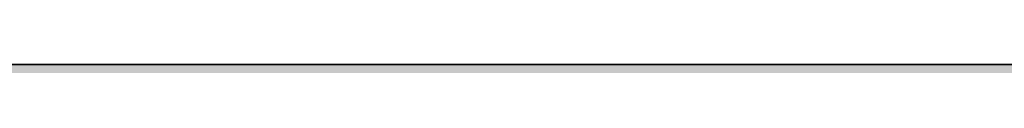
# Model space of a CAD drawing. Units: inches. Extents: x 2091 to 2899, y 967 to 2217.
# Tile 84 of 256: x 2251.24312 to 2251.2787, y 1099.91903 to 1099.91912. Entities that reach past the tile are written whole.
import ezdxf

# ---------------------------------------------------------------- set-up
doc = ezdxf.new("R2010")
doc.units = ezdxf.units.IN
doc.layers.add('A-WALL-PATT', color=141, linetype='Continuous', lineweight=13, true_color=0xadddf7)
doc.layers.add('L-SITE-WALL', color=7, linetype='Continuous', lineweight=35)

msp = doc.modelspace()

# ---------------------------------------------------------------- hatches: boundary and pattern name
at = {"layer": 'A-WALL-PATT'}
h = msp.add_hatch(color=256, dxfattribs=at)
h.dxf.hatch_style = 1
h.paths.add_polyline_path([(2212.143603, 1941.419059), (2387.643603, 1941.419059), (2387.643603, 1824.419059), (2392.143603, 1824.419059), (2392.143603, 1941.419059), (2609.643603, 1941.419059), (2609.643603, 1825.919059), (2614.143603, 1825.919059), (2614.143603, 1941.419059), (2794.143603, 1941.419059), (2794.143603, 1928.762166), (2803.143603, 1928.762166), (2803.143603, 2050.919059), (2203.143603, 2050.919059), (2203.143603, 1900.757859), (2212.143603, 1900.757859)])
h.paths.add_polyline_path([(2212.143603, 1945.919059), (2212.143603, 2041.919059), (2794.143603, 2041.919059), (2794.143603, 1945.919059), (2402.248245, 1945.919059), (2401.102434, 1945.775832), (2398.702434, 1945.775832)], flags=16)
h.paths.add_polyline_path([(2230.229861, 1948.062793), (2227.349861, 1949.502793), (2225.909861, 1951.902793), (2223.989861, 1952.862793), (2223.029861, 1955.262793), (2222.069861, 1959.582793), (2222.069861, 1963.422793), (2223.029861, 1965.662793), (2223.989861, 1965.342793), (2225.58591, 1963.860747), (2226.911533, 1964.957259), (2226.948861, 1965.938793), (2227.778319, 1966.952143), (2228.199916, 1968.878704), (2230.709861, 1964.862793), (2233.589861, 1966.302793), (2233.607309, 1966.331873), (2233.772659, 1964.938205), (2234.633802, 1963.676473), (2235.029861, 1963.902793), (2236.282035, 1965.572358), (2235.989861, 1962.942793), (2237.954512, 1957.540002), (2238.389861, 1957.902793), (2239.215861, 1960.305793), (2238.654565, 1966.38496), (2238.692792, 1966.438069), (2238.840578, 1967.499707), (2238.780291, 1967.687486), (2238.880538, 1967.786763), (2238.666861, 1966.251793), (2239.215861, 1960.305793), (2238.389861, 1957.902793), (2236.949861, 1956.702793), (2234.549861, 1949.982793)], flags=0)
h.paths.add_polyline_path([(2278.011974, 1948.062793), (2276.496427, 1947.873349), (2275.849833, 1947.688608), (2274.651974, 1947.102793)], flags=0)
h.paths.add_polyline_path([(2269.851974, 1955.742793), (2268.276176, 1956.629329), (2270.867302, 1956.348398), (2269.371974, 1958.142793), (2268.714964, 1959.192325), (2270.569833, 1958.728608), (2268.580725, 1961.906087), (2270.811974, 1960.891883), (2270.811974, 1963.422793), (2271.393315, 1964.779256), (2270.291762, 1966.156196), (2271.771974, 1965.662793), (2272.141387, 1966.524757), (2273.929833, 1965.928608), (2275.630385, 1968.054299), (2276.331938, 1966.72186), (2276.520431, 1966.952143), (2276.942029, 1968.878704), (2277.734293, 1967.611082), (2278.139888, 1969.46452), (2279.659124, 1967.033742), (2280.411974, 1966.782793), (2280.949302, 1967.588785), (2281.609833, 1967.368608), (2282.133266, 1968.153758), (2282.349235, 1966.333445), (2282.349849, 1966.332585), (2283.40755, 1968.09542), (2283.712631, 1965.52402), (2284.320221, 1964.633789), (2284.511809, 1964.889239), (2284.234974, 1965.704793), (2284.500472, 1967.318958), (2284.907944, 1965.41742), (2285.396313, 1966.068579), (2285.432833, 1966.290608), (2285.473338, 1966.171279), (2286.353919, 1967.345387), (2286.222007, 1966.158173), (2287.663492, 1968.080154), (2287.713974, 1968.442793), (2288.481599, 1969.016679), (2288.573993, 1968.728897), (2288.917461, 1969.06904), (2288.606833, 1966.837608), (2288.928726, 1963.35131), (2288.934974, 1963.356793), (2288.929731, 1963.340422), (2289.015281, 1962.413869), (2290.111223, 1963.875126), (2290.132833, 1963.942608), (2290.217672, 1964.017058), (2290.111223, 1963.875126), (2289.155833, 1960.891608), (2288.594036, 1959.257227), (2288.571974, 1959.102793), (2289.531974, 1960.542793), (2290.011974, 1962.462793), (2290.19184, 1962.642659), (2289.769833, 1959.688608), (2286.889833, 1957.288608), (2284.489833, 1950.568608), (2283.314658, 1950.046308), (2283.291974, 1949.982793), (2280.290059, 1948.648608), (2281.129833, 1948.648608), (2282.569833, 1948.168608), (2283.204726, 1948.062793), (2278.971974, 1948.062793), (2276.091974, 1949.502793), (2274.651974, 1951.902793), (2272.731974, 1952.862793)], flags=0)
h.paths.add_polyline_path([(2271.158868, 1958.021765), (2272.969833, 1955.848608), (2272.009833, 1960.168608), (2272.009833, 1964.008608), (2272.624426, 1965.442658), (2274.328023, 1963.860747), (2275.653646, 1964.957259), (2275.637743, 1964.53909), (2277.412231, 1966.006888), (2277.032974, 1965.156793), (2276.829924, 1964.975597), (2276.766012, 1963.295014), (2277.449635, 1962.66022), (2279.451974, 1964.862793), (2282.331974, 1966.302793), (2283.529833, 1966.888608), (2283.294512, 1966.770948), (2283.912993, 1963.8847), (2284.899249, 1964.448275), (2284.731974, 1962.942793), (2286.696625, 1957.540002), (2287.131974, 1957.902793), (2287.541913, 1959.095388), (2287.779395, 1958.442311), (2285.682738, 1956.695097), (2285.876503, 1959.795336), (2284.731974, 1962.942793), (2284.899249, 1964.448275), (2283.912993, 1963.8847), (2284.223833, 1962.434116), (2283.424365, 1963.605484), (2281.609833, 1962.568608), (2281.129833, 1960.168608), (2282.089833, 1956.328608), (2283.049833, 1952.968608), (2282.569833, 1950.568608), (2280.169833, 1948.648608), (2279.883316, 1948.791867), (2278.971974, 1948.062793), (2278.971974, 1949.022793), (2278.672313, 1949.397368), (2277.289833, 1950.088608), (2275.849833, 1952.488608), (2273.929833, 1953.448608), (2272.489833, 1954.888608), (2271.921647, 1954.888608), (2271.771974, 1955.262793)], flags=0)
h.paths.add_polyline_path([(2311.994146, 1955.742793), (2312.062717, 1955.674221), (2312.0551, 1955.7085)], flags=0)
h.paths.add_polyline_path([(2331.956146, 1963.951793), (2333.396146, 1965.391793), (2331.077146, 1963.356793), (2330.998603, 1963.111517)], flags=0)
h.paths.add_polyline_path([(2310.554146, 1954.302793), (2307.039807, 1956.279943), (2310.762903, 1955.876284), (2312.474146, 1953.822793), (2313.434146, 1951.422793), (2315.354146, 1950.462793), (2316.794146, 1948.062793), (2317.466146, 1947.726793), (2319.368691, 1947.964611), (2317.754146, 1949.982793), (2317.569531, 1950.610485), (2316.794146, 1951.902793), (2314.874146, 1952.862793), (2313.914146, 1955.262793), (2311.514146, 1958.142793), (2309.375489, 1961.559168), (2311.514146, 1960.337078), (2311.514146, 1961.982793), (2310.604672, 1963.119635), (2311.726605, 1962.47853), (2312.418332, 1964.09256), (2312.255964, 1964.29552), (2313.194146, 1963.982793), (2313.914146, 1965.662793), (2314.646778, 1965.418582), (2315.354146, 1966.302793), (2316.794146, 1967.742793), (2316.157435, 1966.946904), (2317.034111, 1965.28186), (2317.222604, 1965.512143), (2317.777048, 1968.045771), (2318.474111, 1966.72186), (2318.662604, 1966.952143), (2319.084201, 1968.878704), (2321.207049, 1965.482147), (2322.161419, 1966.913702), (2322.554146, 1966.782793), (2322.785988, 1967.130555), (2322.881646, 1966.324293), (2323.312041, 1965.72174), (2323.651289, 1965.891364), (2324.3965, 1967.133382), (2324.656945, 1964.938205), (2324.971986, 1964.476611), (2325.38728, 1967.001499), (2325.940813, 1964.418348), (2327.228929, 1966.135836), (2327.16632, 1965.572358), (2328.059139, 1966.762783), (2328.224576, 1966.247486), (2329.667971, 1967.67691), (2329.664576, 1967.687486), (2329.764823, 1967.786763), (2329.551146, 1966.251793), (2330.100146, 1960.305793), (2329.332814, 1958.07347), (2329.313065, 1957.935225), (2329.634146, 1958.202793), (2330.234146, 1959.102793), (2330.714146, 1961.022793), (2331.034146, 1961.342793), (2330.714146, 1959.102793), (2329.634146, 1958.202793), (2329.274146, 1957.662793), (2327.712112, 1956.361098), (2325.434146, 1949.982793), (2324.333769, 1949.493736), (2323.994146, 1948.542793), (2319.674146, 1946.622793), (2316.794146, 1948.062793), (2315.354146, 1950.462793), (2313.434146, 1951.422793)], flags=0)
h.paths.add_polyline_path([(2321.335684, 1947.952023), (2321.114146, 1948.062793), (2321.114146, 1949.022793), (2319.194146, 1951.422793), (2316.794146, 1959.582793), (2316.663237, 1959.582793), (2315.354146, 1958.142793), (2314.394146, 1958.142793), (2313.148303, 1958.709085), (2312.954146, 1959.582793), (2312.954146, 1960.891883), (2315.834146, 1959.582793), (2316.663237, 1959.582793), (2317.314709, 1960.299412), (2315.030195, 1962.420747), (2316.355818, 1963.517259), (2316.372337, 1963.951615), (2316.470195, 1963.860747), (2317.795818, 1964.957259), (2317.755219, 1963.889687), (2319.175146, 1965.156793), (2319.498407, 1965.881372), (2321.114146, 1965.342793), (2323.235885, 1962.372358), (2325.686349, 1963.772623), (2325.542789, 1962.480576), (2325.198783, 1963.494014), (2324.47851, 1963.082429), (2324.926005, 1960.994116), (2324.078087, 1962.236473), (2322.414791, 1961.286018), (2322.074146, 1959.582793), (2323.034146, 1955.742793), (2323.994146, 1952.382793), (2323.514146, 1949.982793), (2322.142717, 1948.88565), (2322.074146, 1948.542793)], flags=0)
h.paths.add_polyline_path([(2320.207479, 1963.337459), (2320.154146, 1963.422793), (2320.394146, 1963.542793)], flags=0)
h.paths.add_polyline_path([(2353.850527, 1965.8105), (2354.030527, 1965.7505), (2354.330527, 1966.4505), (2354.330527, 1966.9305)], flags=0)
h.paths.add_polyline_path([(2359.020582, 1969.026412), (2359.098382, 1968.901932), (2359.233527, 1969.5195), (2359.233527, 1969.9995)], flags=0)
h.paths.add_polyline_path([(2358.256694, 1966.681672), (2357.983601, 1966.348035), (2358.211267, 1966.146175), (2358.410492, 1966.389568)], flags=0)
h.paths.add_polyline_path([(2357.768473, 1966.058778), (2357.7322, 1965.104967), (2357.751047, 1965.120556), (2357.769527, 1965.6065), (2357.769527, 1966.057843)], flags=0)
h.paths.add_polyline_path([(2359.111527, 1965.3045), (2359.111527, 1964.8245), (2359.844527, 1966.4675), (2359.844527, 1966.9475)], flags=0)
h.paths.add_polyline_path([(2360.223684, 1966.621449), (2360.698527, 1969.3625), (2360.698527, 1969.8425), (2360.210527, 1967.0255), (2360.210527, 1966.6425)], flags=0)
h.paths.add_polyline_path([(2363.450527, 1967.8905), (2363.450527, 1968.3705), (2362.490527, 1966.9305), (2362.656045, 1966.698776)], flags=0)
h.paths.add_polyline_path([(2364.475523, 1966.078826), (2365.850527, 1968.3705), (2365.850527, 1968.8505), (2364.427975, 1966.479581)], flags=0)
h.paths.add_polyline_path([(2366.313527, 1965.8525), (2366.366709, 1965.695829), (2366.802527, 1968.3455), (2366.802527, 1968.8255)], flags=0)
h.paths.add_polyline_path([(2367.16531, 1965.803544), (2367.290527, 1966.9305), (2367.290527, 1967.4105), (2367.102701, 1965.720066)], flags=0)
h.paths.add_polyline_path([(2370.036527, 1959.9735), (2371.013527, 1963.0245), (2371.013527, 1963.5045), (2370.036527, 1960.4535)], flags=0)
h.paths.add_polyline_path([(2371.610527, 1960.2105), (2372.570527, 1961.6505), (2372.570527, 1962.1305), (2371.802527, 1960.9785)], flags=0)
h.paths.add_polyline_path([(2350.873666, 1956.005086), (2351.930527, 1955.8905), (2354.490527, 1953.3305), (2353.850527, 1954.9305), (2351.450527, 1957.8105), (2347.935527, 1963.4255), (2347.935527, 1963.9055), (2351.450527, 1958.2905), (2353.705073, 1955.585046), (2352.890527, 1959.2505), (2352.890527, 1959.7305), (2352.890527, 1961.924786), (2356.730527, 1959.7305), (2358.454471, 1961.626838), (2354.810527, 1965.0105), (2355.030855, 1965.28591), (2358.691091, 1961.88712), (2361.530527, 1965.0105), (2364.376495, 1966.433484), (2364.524394, 1965.186911), (2365.454468, 1963.824181), (2365.881073, 1964.067955), (2365.370527, 1966.4505), (2365.370527, 1966.9305), (2366.810527, 1960.2105), (2366.810527, 1959.7305), (2366.388709, 1952.981409), (2367.770527, 1956.8505), (2368.641225, 1957.576082), (2366.810527, 1962.6105), (2366.810527, 1963.0905), (2368.775179, 1957.68771), (2369.210527, 1958.0505), (2370.001592, 1960.351867), (2369.475232, 1966.052668), (2369.513458, 1966.105777), (2369.514173, 1966.110912), (2369.475232, 1966.532668), (2369.513458, 1966.585777), (2369.614635, 1967.312591), (2369.182527, 1968.6585), (2369.182527, 1969.1385), (2369.600957, 1967.835194), (2369.701204, 1967.934471), (2369.717947, 1968.054743), (2370.145176, 1968.374145), (2369.778707, 1968.011224), (2369.701204, 1967.454471), (2370.468161, 1968.214004), (2369.674936, 1967.265771), (2369.514173, 1966.110912), (2370.036527, 1960.4535), (2370.036527, 1959.9735), (2369.441756, 1958.243191), (2370.650527, 1959.2505), (2371.045821, 1962.017559), (2371.130527, 1962.1305), (2370.650527, 1958.7705), (2367.770527, 1956.3705), (2365.370527, 1949.6505), (2362.079099, 1948.187643), (2363.450527, 1947.7305), (2361.050527, 1947.7305), (2360.090527, 1947.7305), (2357.103861, 1947.357167), (2360.090527, 1948.2105), (2358.170527, 1949.1705), (2356.730527, 1951.5705), (2354.810527, 1952.5305), (2351.930527, 1955.4105)], flags=0)
h.paths.add_polyline_path([(2361.050527, 1948.6905), (2359.130527, 1951.0905), (2356.730527, 1959.2505), (2355.770527, 1959.2505), (2352.890527, 1960.559591), (2352.890527, 1961.444786), (2355.890527, 1959.7305), (2356.730527, 1959.7305), (2356.837194, 1959.367834), (2361.530527, 1964.5305), (2363.248422, 1965.389448), (2364.92531, 1963.041805), (2362.490527, 1961.6505), (2362.063861, 1959.517167), (2362.970527, 1955.8905), (2363.930527, 1952.5305), (2363.930527, 1952.0505), (2363.450527, 1949.6505), (2361.050527, 1947.7305)], flags=0)
h.paths.add_polyline_path([(2359.130527, 1951.5705), (2359.290527, 1951.3705), (2361.050527, 1954.4505), (2361.050527, 1954.9305)], flags=0)
h.paths.add_polyline_path([(2357.219527, 1966.5455), (2356.792527, 1968.8145), (2356.792527, 1969.2945), (2357.219527, 1967.0255)], flags=0)
h.paths.add_polyline_path([(2361.050527, 1954.4505), (2361.530527, 1958.7705), (2361.530527, 1959.2505), (2361.050527, 1954.9305)], flags=0)
h.paths.add_polyline_path([(2402.548287, 1948.486076), (2402.302434, 1948.415832), (2402.590434, 1948.415832)], flags=0)
h.paths.add_polyline_path([(2394.142434, 1956.095832), (2395.685052, 1954.553214), (2396.720495, 1953.970679), (2396.062434, 1955.615832), (2395.241381, 1956.601096), (2395.878904, 1956.441715), (2395.102434, 1959.935832), (2395.102434, 1963.775832), (2396.062434, 1966.015832), (2397.022434, 1965.695832), (2398.618483, 1964.213787), (2399.944106, 1965.310299), (2399.981434, 1966.291832), (2400.810891, 1967.305183), (2401.232489, 1969.231744), (2403.537949, 1965.543008), (2403.941984, 1967.389316), (2404.702434, 1967.135832), (2405.460328, 1966.07478), (2406.622434, 1966.655832), (2406.639882, 1966.684913), (2406.805232, 1965.291245), (2406.925694, 1965.114746), (2407.342434, 1964.975832), (2407.874326, 1965.77367), (2408.1691, 1964.398055), (2409.314608, 1965.925398), (2409.217458, 1965.051054), (2409.445232, 1963.131245), (2410.306374, 1961.869513), (2410.702434, 1962.095832), (2411.442269, 1963.082279), (2411.165434, 1963.897832), (2411.616426, 1966.639757), (2411.725365, 1966.791109), (2411.873151, 1967.852747), (2411.812864, 1968.040526), (2411.913111, 1968.139803), (2411.699434, 1966.604832), (2412.248434, 1960.658832), (2413.225434, 1963.709832), (2414.3779, 1964.72116), (2414.513151, 1965.692747), (2414.452864, 1965.880526), (2414.553111, 1965.979803), (2414.3779, 1964.72116), (2414.519817, 1964.845697), (2414.365365, 1964.631109), (2414.339434, 1964.444832), (2414.888434, 1958.498832), (2414.062434, 1956.095832), (2412.622434, 1954.895832), (2410.17137, 1948.032854), (2410.016719, 1948.084404), (2405.902434, 1946.255832), (2405.902434, 1947.215832), (2405.204252, 1948.08856), (2404.222434, 1948.415832), (2403.262434, 1948.415832), (2400.382434, 1949.855832), (2399.662434, 1951.055832), (2397.982434, 1952.735832), (2397.022434, 1953.215832), (2395.685052, 1954.553214), (2392.656776, 1956.256908)], flags=0)
h.paths.add_polyline_path([(2409.08565, 1964.407441), (2409.130363, 1964.275715), (2409.262434, 1964.495832)], flags=0)
h.paths.add_polyline_path([(2397.742434, 1961.615832), (2398.702434, 1963.855832), (2399.662434, 1963.535832), (2401.426563, 1965.740994), (2401.791415, 1966.5588), (2402.071434, 1965.070832), (2402.835507, 1964.393367), (2403.262398, 1964.9149), (2403.338119, 1964.771086), (2402.615516, 1963.976223), (2402.498612, 1960.902238), (2403.542997, 1959.932452), (2404.413203, 1960.889679), (2404.702434, 1962.335832), (2407.916347, 1964.172354), (2409.520211, 1961.926944), (2410.987085, 1957.893042), (2411.422434, 1958.255832), (2412.047964, 1960.075625), (2412.410341, 1959.079088), (2411.675621, 1958.466821), (2411.662434, 1958.255832), (2411.62607, 1958.425529), (2409.982434, 1957.055832), (2407.582434, 1950.335832), (2403.262434, 1948.415832), (2403.262434, 1949.375832), (2401.342434, 1951.775832), (2399.416508, 1958.323981), (2397.742434, 1959.084923), (2397.742434, 1959.970118), (2397.102434, 1960.335832), (2397.742434, 1960.044923)], flags=0)
h.paths.add_polyline_path([(2405.902434, 1952.975832), (2405.950434, 1953.407832), (2406.016719, 1953.175832)], flags=0)
h.paths.add_polyline_path([(2449.817778, 1967.114014), (2449.752323, 1967.135832), (2449.793703, 1967.077901)], flags=0)
h.paths.add_polyline_path([(2451.697696, 1966.61812), (2451.740895, 1966.690118), (2451.692051, 1966.665696)], flags=0)
h.paths.add_polyline_path([(2454.343628, 1965.737572), (2455.752323, 1967.615832), (2455.992323, 1968.095832), (2454.364497, 1965.925398)], flags=0)
h.paths.add_polyline_path([(2457.547323, 1968.863832), (2457.787323, 1969.343832), (2457.054323, 1968.795832), (2457.007622, 1968.460345)], flags=0)
h.paths.add_polyline_path([(2456.921784, 1967.856662), (2456.802238, 1968.229016), (2456.723, 1967.659803)], flags=0)
h.paths.add_polyline_path([(2457.302323, 1967.376832), (2457.542323, 1967.856832), (2456.810323, 1966.839832), (2456.740516, 1966.700218), (2456.749021, 1966.608105)], flags=0)
h.paths.add_polyline_path([(2458.275323, 1963.709832), (2458.155343, 1963.335153), (2460.354323, 1965.264832), (2460.594323, 1965.744832)], flags=0)
h.paths.add_polyline_path([(2458.392323, 1962.815832), (2458.364088, 1962.618185), (2459.592323, 1964.255832), (2459.832323, 1964.735832)], flags=0)
h.paths.add_polyline_path([(2459.352323, 1962.815832), (2459.272323, 1962.495832), (2460.072323, 1963.295832), (2460.312323, 1963.775832)], flags=0)
h.paths.add_polyline_path([(2458.680323, 1960.607832), (2458.632323, 1960.415832), (2459.592323, 1961.855832), (2459.832323, 1962.335832)], flags=0)
h.paths.add_polyline_path([(2437.83817, 1956.24265), (2439.192323, 1956.095832), (2441.352323, 1953.935832), (2440.872323, 1955.135832), (2438.472323, 1958.015832), (2438.071563, 1958.656023), (2438.712323, 1958.495832), (2440.639596, 1956.183105), (2439.912323, 1959.455832), (2439.912323, 1963.295832), (2441.352323, 1966.655832), (2441.592323, 1967.135832), (2441.112323, 1966.015832), (2442.072323, 1965.695832), (2443.988993, 1968.09167), (2444.241323, 1966.750832), (2444.916801, 1966.15192), (2445.676574, 1967.080136), (2446.255323, 1969.724832), (2446.495323, 1970.204832), (2446.282379, 1969.231744), (2447.362672, 1967.503275), (2447.720323, 1969.567832), (2447.960323, 1970.047832), (2447.48548, 1967.306781), (2448.792323, 1965.215832), (2448.472323, 1964.863832), (2448.552323, 1964.735832), (2451.452051, 1966.185696), (2451.615122, 1964.811245), (2452.307917, 1963.796172), (2453.234505, 1964.325651), (2454.072323, 1960.415832), (2453.628687, 1953.317651), (2454.792323, 1956.575832), (2455.032323, 1957.055832), (2455.718835, 1957.627926), (2453.832323, 1962.815832), (2453.940966, 1963.793615), (2453.335323, 1965.577832), (2453.824323, 1968.550832), (2454.064323, 1969.030832), (2453.575323, 1966.057832), (2454.040333, 1964.687919), (2453.832323, 1962.815832), (2455.718835, 1957.627926), (2456.367207, 1958.168235), (2457.058323, 1960.178832), (2457.298323, 1960.658832), (2456.472323, 1958.255832), (2457.717729, 1959.29367), (2457.672323, 1958.975832), (2454.889951, 1956.657188), (2453.614142, 1953.084923), (2453.592323, 1952.735832), (2453.352323, 1952.255832), (2453.359596, 1952.372196), (2452.632323, 1950.335832), (2452.392323, 1949.855832), (2449.203752, 1948.43869), (2450.712323, 1947.935832), (2448.072323, 1947.935832), (2447.112323, 1947.935832), (2444.552323, 1947.615832), (2447.199596, 1948.372196), (2445.192323, 1949.375832), (2443.752323, 1951.775832), (2441.832323, 1952.735832), (2438.952323, 1955.615832)], flags=0)
h.paths.add_polyline_path([(2443.992323, 1959.935832), (2444.040323, 1959.772632), (2444.121554, 1959.861986)], flags=0)
h.paths.add_polyline_path([(2442.912323, 1959.935832), (2443.032323, 1959.935832), (2442.445657, 1960.202499)], flags=0)
h.paths.add_polyline_path([(2444.982943, 1965.019677), (2445.279323, 1965.264832), (2445.519323, 1965.744832), (2444.993996, 1965.310299)], flags=0)
h.paths.add_polyline_path([(2446.133323, 1965.029832), (2446.330366, 1965.471499), (2444.970323, 1964.257832), (2444.730323, 1963.777832)], flags=0)
h.paths.add_polyline_path([(2442.792323, 1959.455832), (2443.752323, 1959.455832), (2446.152323, 1951.295832), (2446.412323, 1951.750832), (2446.392323, 1951.775832), (2448.080599, 1954.730315), (2448.552323, 1958.975832), (2441.832323, 1965.215832), (2442.154946, 1965.619111), (2448.792323, 1959.455832), (2448.312323, 1955.135832), (2448.072323, 1954.655832), (2446.412323, 1951.750832), (2448.312323, 1949.375832), (2448.312323, 1948.415832), (2450.540895, 1950.19869), (2450.952323, 1952.255832), (2449.992323, 1955.615832), (2449.032323, 1959.455832), (2449.512323, 1961.855832), (2449.752323, 1962.335832), (2449.674904, 1961.948736), (2452.994505, 1963.845651), (2453.064414, 1963.519409), (2452.884611, 1963.782854), (2449.674904, 1961.948736), (2449.272323, 1959.935832), (2450.232323, 1956.095832), (2451.192323, 1952.735832), (2450.712323, 1950.335832), (2450.472323, 1949.855832), (2448.072323, 1947.935832), (2448.072323, 1948.535832), (2445.432323, 1949.855832), (2443.992323, 1952.255832), (2442.072323, 1953.215832), (2441.112323, 1955.615832), (2440.152323, 1959.935832), (2440.152323, 1960.655832)], flags=0)
h.paths.add_polyline_path([(2456.692323, 1966.985832), (2457.608323, 1968.080832), (2457.848323, 1968.560832), (2456.932323, 1967.465832)], flags=0)
h.paths.add_polyline_path([(2489.89657, 1966.580241), (2489.942948, 1966.189347), (2490.747488, 1967.530248), (2491.319122, 1968.951161)], flags=0)
h.paths.add_polyline_path([(2473.562471, 1956.407131), (2477.139981, 1956.019257), (2476.955333, 1956.240834), (2475.108049, 1957.280108), (2476.347488, 1956.970248), (2475.186901, 1958.824216), (2476.919122, 1958.391161), (2475.411642, 1960.799269), (2477.787488, 1959.719339), (2477.787488, 1962.250248), (2477.637399, 1962.43786), (2477.82255, 1962.332059), (2478.359122, 1963.58406), (2478.359122, 1963.671161), (2477.324348, 1964.964628), (2478.714826, 1964.501135), (2479.319122, 1965.911161), (2480.279122, 1965.591161), (2481.783965, 1967.472214), (2482.116488, 1965.705248), (2482.880562, 1965.027782), (2483.209305, 1965.429408), (2483.220169, 1965.71509), (2483.07594, 1965.989022), (2483.711762, 1966.765808), (2484.130488, 1968.679248), (2484.702122, 1970.100161), (2484.489177, 1969.127072), (2486.502904, 1965.905109), (2487.387488, 1965.610248), (2488.153419, 1966.759144), (2488.717017, 1965.970108), (2489.200086, 1966.211642), (2489.330671, 1965.110992), (2490.393905, 1963.622465), (2490.660765, 1963.774956), (2490.493905, 1964.553636), (2490.923063, 1963.924841), (2491.319122, 1964.151161), (2491.333389, 1964.170183), (2491.210488, 1964.532248), (2491.281756, 1964.965537), (2491.425789, 1964.293383), (2494.076476, 1967.827632), (2494.497918, 1966.514942), (2494.598165, 1966.614218), (2494.689488, 1967.270248), (2495.106748, 1967.582196), (2495.129839, 1967.748075), (2495.069552, 1967.935854), (2495.169799, 1968.035131), (2495.031777, 1967.043632), (2495.753818, 1967.758684), (2494.982053, 1966.686437), (2494.956122, 1966.500161), (2495.479021, 1960.836851), (2495.910488, 1962.184248), (2496.482122, 1963.605161), (2496.072694, 1962.326589), (2496.768904, 1962.937536), (2496.599122, 1962.711161), (2496.119122, 1959.351161), (2496.732873, 1960.271787), (2496.987488, 1961.290248), (2497.559122, 1962.711161), (2497.079122, 1960.791161), (2496.507488, 1959.370248), (2495.547488, 1957.930248), (2492.758842, 1955.606376), (2490.839122, 1950.231161), (2490.267488, 1948.810248), (2485.947488, 1946.890248), (2483.067488, 1948.330248), (2481.627488, 1950.730248), (2479.707488, 1951.690248), (2476.827488, 1954.570248)], flags=0)
h.paths.add_polyline_path([(2485.576973, 1948.313392), (2485.559122, 1948.311161), (2485.578758, 1948.311161)], flags=0)
h.paths.add_polyline_path([(2478.645063, 1954.551161), (2478.109042, 1956.963257), (2479.319122, 1955.511161), (2480.279122, 1953.111161), (2482.199122, 1952.151161), (2483.639122, 1949.751161), (2486.519122, 1948.311161), (2486.519122, 1949.271161), (2484.739307, 1951.49593), (2484.027488, 1950.250248), (2481.627488, 1958.410248), (2482.375148, 1959.232673), (2482.199122, 1959.831161), (2483.197572, 1960.929456), (2479.707488, 1964.170248), (2480.603358, 1965.290085), (2481.875171, 1964.109115), (2482.666387, 1964.763582), (2482.615359, 1963.421798), (2482.989199, 1963.074661), (2484.008488, 1963.984248), (2484.683606, 1965.497507), (2484.580122, 1965.405161), (2485.357268, 1967.147113), (2485.120645, 1965.781197), (2486.427488, 1963.690248), (2488.145383, 1964.549195), (2489.822271, 1962.201552), (2490.747488, 1962.730248), (2491.999662, 1964.399813), (2492.076046, 1965.087265), (2492.212892, 1964.684119), (2492.485374, 1965.047429), (2492.279122, 1963.191161), (2494.243773, 1957.78837), (2494.562503, 1958.053978), (2494.933488, 1959.133248), (2495.505122, 1960.554161), (2494.679122, 1958.151161), (2494.107488, 1956.730248), (2494.562503, 1958.053978), (2493.408544, 1957.092345), (2491.707488, 1961.770248), (2491.999662, 1964.399813), (2490.747488, 1962.730248), (2487.71203, 1960.9957), (2487.479122, 1959.831161), (2488.439122, 1955.991161), (2489.399122, 1952.631161), (2488.919122, 1950.231161), (2488.576918, 1949.957397), (2488.347488, 1948.810248), (2487.651715, 1948.253629), (2487.479122, 1948.311161), (2486.519122, 1948.311161), (2483.639122, 1949.751161), (2482.199122, 1952.151161), (2480.279122, 1953.111161), (2478.839122, 1954.551161)], flags=0)
h.paths.add_polyline_path([(2526.648252, 1966.987524), (2526.517343, 1967.031161), (2526.600102, 1966.915298)], flags=0)
h.paths.add_polyline_path([(2528.47064, 1966.446656), (2528.574486, 1966.619732), (2528.457071, 1966.561025)], flags=0)
h.paths.add_polyline_path([(2534.133343, 1967.496161), (2534.156685, 1967.542845), (2534.059841, 1967.408296)], flags=0)
h.paths.add_polyline_path([(2536.161923, 1964.0506), (2535.157343, 1962.711161), (2535.100872, 1962.315866), (2536.117343, 1963.671161), (2536.420532, 1964.277539)], flags=0)
h.paths.add_polyline_path([(2535.157343, 1959.831161), (2536.117343, 1961.271161), (2536.597343, 1962.231161), (2535.253343, 1960.215161)], flags=0)
h.paths.add_polyline_path([(2513.249035, 1956.284796), (2516.221181, 1955.962555), (2514.997343, 1957.431161), (2514.195823, 1958.711541), (2515.477343, 1958.391161), (2516.931888, 1956.645706), (2516.437343, 1958.871161), (2516.437343, 1962.711161), (2516.872692, 1963.726974), (2515.346434, 1965.634797), (2517.397343, 1964.951161), (2517.877343, 1966.071161), (2518.357343, 1967.031161), (2517.877343, 1965.911161), (2518.837343, 1965.591161), (2520.48659, 1967.652719), (2520.766343, 1966.166161), (2521.530417, 1965.488695), (2521.781443, 1965.795375), (2521.800911, 1966.307268), (2521.477804, 1966.920936), (2521.246343, 1967.126161), (2521.177701, 1967.490913), (2521.477804, 1966.920936), (2522.010417, 1966.448695), (2522.257386, 1966.750417), (2522.780343, 1969.140161), (2523.260343, 1970.100161), (2523.047398, 1969.127072), (2524.673132, 1966.525897), (2526.037343, 1966.071161), (2526.795238, 1965.010108), (2527.977071, 1965.601025), (2528.140141, 1964.226573), (2528.66459, 1963.458159), (2529.388616, 1963.871888), (2529.329665, 1964.14699), (2529.481284, 1963.924841), (2529.877343, 1964.151161), (2529.98401, 1964.293383), (2529.789053, 1965.20318), (2530.0624, 1964.397903), (2532.802483, 1968.051347), (2533.147773, 1966.975854), (2533.24802, 1967.075131), (2533.339343, 1967.731161), (2533.672848, 1967.980493), (2533.72802, 1968.035131), (2533.514343, 1966.500161), (2534.024718, 1960.972496), (2534.560343, 1962.645161), (2535.040343, 1963.605161), (2534.063343, 1960.554161), (2533.237343, 1958.151161), (2534.288154, 1959.026836), (2534.197343, 1958.391161), (2531.512597, 1956.153872), (2529.397343, 1950.231161), (2528.917343, 1949.271161), (2526.448772, 1948.174018), (2527.477343, 1947.831161), (2530.357343, 1947.351161), (2524.597343, 1947.351161), (2521.717343, 1948.791161), (2520.277343, 1951.191161), (2518.357343, 1952.151161), (2515.477343, 1955.031161)], flags=0)
h.paths.add_polyline_path([(2523.93476, 1967.190308), (2523.619512, 1966.483689), (2523.7705, 1966.242109)], flags=0)
h.paths.add_polyline_path([(2518.837343, 1953.111161), (2517.877343, 1955.511161), (2516.884983, 1959.976779), (2516.917343, 1959.96207), (2516.917343, 1962.025446), (2520.757343, 1959.831161), (2522.024949, 1961.225527), (2518.357343, 1964.631161), (2519.002589, 1965.437718), (2520.433392, 1964.109115), (2521.30112, 1964.826871), (2521.245157, 1963.355333), (2525.638307, 1959.27598), (2526.037343, 1961.271161), (2529.397343, 1963.191161), (2530.649517, 1964.860726), (2530.66472, 1964.99755), (2530.691956, 1964.917311), (2531.087778, 1965.445074), (2530.945985, 1964.168944), (2530.691956, 1964.917311), (2529.397343, 1963.191161), (2526.362504, 1961.456967), (2526.037343, 1959.831161), (2526.997343, 1955.991161), (2527.957343, 1952.631161), (2527.477343, 1950.231161), (2527.134486, 1949.956875), (2526.973928, 1949.154087), (2526.697343, 1949.031161), (2524.597343, 1947.351161), (2524.597343, 1948.311161), (2524.277343, 1948.711161), (2522.197343, 1949.751161), (2520.757343, 1952.151161)], flags=0)
h.paths.add_polyline_path([(2520.277343, 1958.871161), (2520.853343, 1959.504761), (2523.157343, 1951.671161), (2524.613895, 1954.220126), (2524.597343, 1954.071161), (2522.677343, 1950.711161)], flags=0)
h.paths.add_polyline_path([(2559.37091, 1966.311161), (2559.398411, 1966.324911), (2559.401943, 1966.345296)], flags=0)
h.paths.add_polyline_path([(2549.77091, 1957.191161), (2552.65091, 1954.311161), (2552.133987, 1955.603468), (2550.61091, 1957.431161), (2547.09591, 1963.046161), (2545.77591, 1965.206161), (2549.29091, 1959.591161), (2551.69091, 1956.711161), (2550.792933, 1960.752059), (2550.73091, 1960.780251), (2550.73091, 1964.871161), (2551.69091, 1967.111161), (2552.65091, 1966.791161), (2554.246959, 1965.309115), (2555.034252, 1965.960337), (2555.581671, 1966.644612), (2555.60991, 1967.387161), (2556.439368, 1968.400511), (2556.860966, 1970.327072), (2559.37091, 1966.311161), (2560.69091, 1964.151161), (2562.408805, 1965.010108), (2561.65091, 1966.071161), (2560.33091, 1968.231161), (2561.758497, 1966.23254), (2562.347213, 1967.115614), (2562.433709, 1966.386573), (2563.127798, 1965.369604), (2563.57091, 1965.591161), (2563.588359, 1965.620241), (2563.362543, 1967.52354), (2563.722489, 1965.843792), (2565.060001, 1968.072979), (2564.732862, 1965.128722), (2565.117577, 1963.333383), (2567.444622, 1966.436109), (2567.315615, 1967.833328), (2567.353841, 1967.886437), (2567.501627, 1968.948075), (2567.44134, 1969.135854), (2567.541587, 1969.235131), (2567.32791, 1967.700161), (2567.87691, 1961.754161), (2568.746689, 1964.470327), (2568.635615, 1965.673328), (2568.673841, 1965.726437), (2568.821627, 1966.788075), (2568.76134, 1966.975854), (2568.861587, 1967.075131), (2568.64791, 1965.540161), (2568.726127, 1964.693026), (2568.85391, 1964.805161), (2568.746689, 1964.470327), (2568.817236, 1963.706261), (2568.97091, 1963.911161), (2568.866075, 1963.17731), (2569.19691, 1959.594161), (2568.37091, 1957.191161), (2566.93091, 1955.991161), (2564.620272, 1949.521373), (2564.65091, 1949.511161), (2564.616625, 1949.511161), (2564.53091, 1949.271161), (2560.21091, 1947.351161), (2557.33091, 1948.791161), (2556.045196, 1950.934018), (2556.01091, 1950.951161), (2555.856625, 1951.208303), (2553.97091, 1952.151161), (2551.09091, 1955.031161), (2546.650144, 1957.529515)], flags=0)
h.paths.add_polyline_path([(2567.025794, 1959.33023), (2567.035007, 1959.304895), (2567.05091, 1959.351161)], flags=0)
h.paths.add_polyline_path([(2551.968287, 1962.518374), (2553.01091, 1964.951161), (2553.97091, 1964.631161), (2555.566959, 1963.149115), (2556.892583, 1964.245627), (2556.92991, 1965.227161), (2557.143984, 1965.488695), (2556.420066, 1966.130557), (2556.391421, 1966.104995), (2556.37991, 1966.166161), (2556.420066, 1966.130557), (2556.95191, 1966.605161), (2557.092139, 1966.919478), (2557.570875, 1966.010228), (2557.759368, 1966.240511), (2557.41791, 1964.680161), (2556.892583, 1964.245627), (2556.807089, 1961.997566), (2560.69091, 1958.391161), (2560.635526, 1957.892699), (2560.81091, 1957.191161), (2561.77091, 1953.831161), (2561.29091, 1951.431161), (2559.110423, 1949.68677), (2559.156484, 1949.629193), (2563.02652, 1951.349209), (2562.61091, 1949.271161), (2560.21091, 1947.351161), (2560.21091, 1948.311161), (2559.25091, 1949.511161), (2558.89091, 1949.511161), (2558.89091, 1949.961161), (2558.29091, 1950.711161), (2558.053701, 1951.517672), (2556.97091, 1952.871161), (2555.06788, 1959.341464), (2552.05091, 1961.065446), (2552.05091, 1962.471161)], flags=0)
h.paths.add_polyline_path([(2588.330049, 1958.391161), (2588.610248, 1958.110962), (2588.553362, 1958.366949)], flags=0)
h.paths.add_polyline_path([(2594.745454, 1950.493086), (2593.957532, 1953.172022), (2593.130049, 1954.551161), (2591.210049, 1955.511161), (2590.250049, 1957.911161), (2588.309033, 1960.240379), (2586.177306, 1961.209346), (2587.850049, 1960.791161), (2587.253416, 1961.744246), (2588.441314, 1961.065446), (2588.441314, 1962.655528), (2588.421679, 1962.665345), (2588.441314, 1962.711161), (2586.914038, 1964.620256), (2588.877086, 1963.727962), (2589.290049, 1964.69154), (2589.290049, 1966.071161), (2590.250049, 1968.311161), (2591.210049, 1967.991161), (2592.806098, 1966.509115), (2594.131721, 1967.605627), (2594.169049, 1968.587161), (2594.998506, 1969.600511), (2595.420104, 1971.527072), (2597.930049, 1967.511161), (2600.810049, 1968.951161), (2600.827497, 1968.980241), (2600.992847, 1967.586573), (2601.853989, 1966.324841), (2602.107143, 1966.4695), (2602.236354, 1967.255069), (2602.356715, 1966.693383), (2603.502223, 1968.220726), (2603.210049, 1965.591161), (2605.1747, 1960.18837), (2605.506891, 1960.465196), (2605.026019, 1965.673328), (2605.064245, 1965.726437), (2605.212031, 1966.788075), (2605.151744, 1966.975854), (2605.251991, 1967.075131), (2605.343314, 1967.731161), (2605.952905, 1968.186898), (2605.874753, 1969.033328), (2605.912979, 1969.086437), (2606.060766, 1970.148075), (2606.000479, 1970.335854), (2606.100725, 1970.435131), (2605.887049, 1968.900161), (2606.436049, 1962.954161), (2605.610049, 1960.551161), (2605.997036, 1960.87365), (2606.564314, 1962.645161), (2608.241494, 1964.116941), (2608.010049, 1963.191161), (2607.050049, 1961.751161), (2606.631486, 1961.402358), (2606.201314, 1958.391161), (2603.321314, 1955.991161), (2600.921314, 1949.271161), (2596.601314, 1947.351161), (2593.721314, 1948.791161), (2592.857314, 1950.231161), (2592.650049, 1950.231161)], flags=0)
h.paths.add_polyline_path([(2596.601314, 1947.351161), (2596.601314, 1948.311161), (2594.681314, 1950.711161), (2596.154954, 1953.290029), (2595.530049, 1954.071161), (2593.199226, 1961.995957), (2592.65134, 1962.504708), (2591.780151, 1963.002531), (2593.282987, 1964.245627), (2593.320314, 1965.227161), (2594.149772, 1966.240511), (2594.57137, 1968.167072), (2596.182651, 1965.589023), (2596.951273, 1966.434508), (2598.041314, 1966.071161), (2598.799209, 1965.010108), (2599.961314, 1965.591161), (2599.978763, 1965.620241), (2600.144113, 1964.226573), (2601.005255, 1962.964841), (2601.401314, 1963.191161), (2602.653488, 1964.860726), (2602.361314, 1962.231161), (2603.792748, 1958.294719), (2601.977644, 1953.212427), (2601.946208, 1952.709453), (2599.468755, 1951.608363), (2599.001314, 1949.271161)], flags=0)
h.paths.add_polyline_path([(2597.561314, 1958.871161), (2597.670966, 1959.419419), (2597.595054, 1958.736204)], flags=0)
h.paths.add_polyline_path([(2623.666305, 1961.254375), (2625.519163, 1960.791161), (2624.965544, 1961.675533), (2627.199163, 1960.660251), (2627.199163, 1961.151161), (2626.959163, 1962.231161), (2626.959163, 1963.491161), (2625.582321, 1965.212213), (2626.959163, 1964.425446), (2626.959163, 1965.831161), (2626.869163, 1965.861161), (2627.919163, 1968.311161), (2628.879163, 1967.991161), (2630.475212, 1966.509115), (2631.800835, 1967.605627), (2631.838163, 1968.587161), (2632.667621, 1969.600511), (2633.089218, 1971.527072), (2635.599163, 1967.511161), (2638.479163, 1968.951161), (2638.496611, 1968.980241), (2638.661961, 1967.586573), (2639.176273, 1966.833011), (2639.780216, 1967.839582), (2640.02583, 1966.693383), (2641.171337, 1968.220726), (2640.879163, 1965.591161), (2641.114265, 1964.94463), (2641.411337, 1965.340726), (2641.308099, 1964.411586), (2642.843814, 1960.18837), (2643.279163, 1960.551161), (2644.084736, 1962.894736), (2643.783867, 1966.153328), (2643.806834, 1966.185237), (2643.600676, 1968.418053), (2643.522812, 1968.660581), (2643.72988, 1970.148075), (2643.669593, 1970.335854), (2643.76984, 1970.435131), (2643.556163, 1968.900161), (2643.600676, 1968.418053), (2643.909593, 1967.455854), (2644.00984, 1967.555131), (2643.811743, 1966.132079), (2644.105163, 1962.954161), (2644.238773, 1961.350836), (2644.719163, 1961.751161), (2645.032853, 1962.221695), (2645.322163, 1963.125161), (2646.07642, 1963.787047), (2645.032853, 1962.221695), (2644.345163, 1960.074161), (2643.519163, 1957.671161), (2642.079163, 1956.471161), (2639.719612, 1949.864419), (2639.875527, 1949.838433), (2635.359163, 1947.831161), (2632.479163, 1949.271161), (2631.039163, 1951.671161), (2629.119163, 1952.631161), (2628.159163, 1955.031161), (2625.759163, 1957.911161)], flags=0)
h.paths.add_polyline_path([(2627.816306, 1956.574018), (2627.373708, 1958.565706), (2626.376306, 1959.762589), (2627.199163, 1959.351161), (2627.373708, 1958.565706), (2627.919163, 1957.911161), (2628.879163, 1955.511161), (2630.799163, 1954.551161), (2632.239163, 1952.151161), (2633.315025, 1951.613229), (2631.039163, 1959.351161), (2631.49783, 1959.855694), (2630.799163, 1962.231161), (2631.449867, 1962.946935), (2630.715212, 1963.629115), (2632.040835, 1964.725627), (2632.078163, 1965.707161), (2632.292237, 1965.968695), (2631.705339, 1966.489067), (2633.136441, 1967.766144), (2633.329218, 1968.647072), (2634.674718, 1966.494272), (2635.208465, 1967.081393), (2636.799163, 1966.551161), (2637.676404, 1967.867023), (2638.993946, 1966.022465), (2639.705345, 1966.428979), (2641.119163, 1959.831161), (2640.930072, 1956.805706), (2639.439163, 1952.631161), (2638.227456, 1952.092624), (2637.759163, 1949.751161), (2635.359163, 1947.831161), (2635.359163, 1948.791161), (2633.439163, 1951.191161), (2633.315025, 1951.613229), (2632.239163, 1952.151161), (2630.799163, 1954.551161), (2628.879163, 1955.511161)], flags=0)
h.paths.add_polyline_path([(2637.759163, 1953.831161), (2637.279163, 1955.511161), (2636.319163, 1959.351161), (2636.799163, 1961.751161), (2639.233946, 1963.142465), (2637.557058, 1965.490108), (2638.738891, 1966.081025), (2638.901961, 1964.706573), (2639.763104, 1963.444841), (2636.799163, 1961.751161), (2636.532496, 1960.417827), (2637.039163, 1958.391161), (2637.999163, 1955.031161)], flags=0)
h.paths.add_polyline_path([(2668.567407, 1951.431161), (2667.607407, 1953.831161), (2665.207407, 1956.711161), (2662.293903, 1961.365307), (2665.447407, 1959.591161), (2666.647407, 1958.391161), (2666.647407, 1959.975161), (2666.058317, 1960.68207), (2666.647407, 1960.345446), (2666.647407, 1961.991161), (2666.70009, 1962.114087), (2666.407407, 1963.431161), (2666.407407, 1967.271161), (2667.367407, 1969.511161), (2668.327407, 1969.191161), (2669.923457, 1967.709115), (2671.24908, 1968.805627), (2671.286407, 1969.787161), (2672.115865, 1970.800511), (2672.537463, 1972.727072), (2675.047407, 1968.711161), (2677.927407, 1970.151161), (2677.944856, 1970.180241), (2678.110206, 1968.786573), (2678.971348, 1967.524841), (2679.367407, 1967.751161), (2680.619581, 1969.420726), (2680.327407, 1966.791161), (2682.292059, 1961.38837), (2682.727407, 1961.751161), (2683.358306, 1963.586571), (2683.232112, 1964.953328), (2683.270338, 1965.006437), (2683.393215, 1965.889138), (2683.359969, 1966.249215), (2683.357837, 1966.255854), (2683.359229, 1966.257232), (2682.992112, 1970.233328), (2683.030338, 1970.286437), (2683.178124, 1971.348075), (2683.117837, 1971.535854), (2683.218084, 1971.635131), (2683.004407, 1970.100161), (2683.359229, 1966.257232), (2683.458084, 1966.355131), (2683.393215, 1965.889138), (2683.413908, 1965.665023), (2684.42381, 1966.872275), (2683.553407, 1964.154161), (2683.358306, 1963.586571), (2683.793407, 1958.874161), (2682.967407, 1956.471161), (2681.527407, 1955.271161), (2680.109226, 1951.300251), (2680.084933, 1950.911573), (2679.976846, 1950.929587), (2679.127407, 1948.551161), (2674.807407, 1946.631161), (2671.927407, 1948.071161), (2670.487407, 1950.471161)], flags=0)
h.paths.add_polyline_path([(2671.935683, 1953.227023), (2671.687407, 1953.351161), (2670.247407, 1955.751161), (2668.327407, 1956.711161), (2667.356741, 1959.137827), (2669.527407, 1958.151161), (2670.487407, 1958.151161), (2671.479407, 1959.242361), (2670.684402, 1961.94538), (2668.889599, 1963.611982), (2667.307407, 1964.331161), (2668.567407, 1963.911161), (2668.830937, 1964.240572), (2670.247407, 1963.431161), (2672.42214, 1965.823367), (2672.777463, 1967.447072), (2673.234074, 1966.716494), (2674.411919, 1968.012124), (2673.980564, 1965.522109), (2675.287407, 1963.431161), (2675.554074, 1963.564494), (2675.932407, 1965.456161), (2676.247407, 1965.351161), (2677.005302, 1964.290108), (2678.167407, 1964.871161), (2679.607407, 1967.271161), (2680.327407, 1963.911161), (2680.306552, 1963.57748), (2680.347242, 1963.457607), (2680.859581, 1964.140726), (2680.567407, 1961.511161), (2681.103624, 1960.036566), (2678.887407, 1953.831161), (2677.092478, 1953.033414), (2677.687407, 1950.951161), (2677.207407, 1948.551161), (2674.807407, 1946.631161), (2674.807407, 1947.591161), (2672.887407, 1949.991161)], flags=0)
h.paths.add_polyline_path([(2673.98455, 1951.911161), (2674.567407, 1952.931161), (2674.567407, 1951.911161), (2676.967407, 1953.831161), (2677.447407, 1956.231161), (2676.487407, 1959.591161), (2676.247407, 1960.551161), (2679.729589, 1962.540979), (2680.059267, 1961.002484), (2679.211348, 1962.244841), (2676.247407, 1960.551161), (2676.487407, 1959.591161), (2677.447407, 1956.231161), (2676.967407, 1953.831161), (2674.567407, 1951.911161)], flags=0)
h.paths.add_polyline_path([(2707.479283, 1952.814651), (2706.519283, 1955.214651), (2705.559283, 1959.534651), (2705.559283, 1963.374651), (2706.519283, 1965.614651), (2707.479283, 1965.294651), (2709.075332, 1963.812605), (2710.400956, 1964.909117), (2710.438283, 1965.890651), (2711.267741, 1966.904001), (2711.689338, 1968.830563), (2714.199283, 1964.814651), (2717.079283, 1966.254651), (2717.096731, 1966.283731), (2717.262082, 1964.890063), (2718.123224, 1963.628331), (2718.519283, 1963.854651), (2719.771457, 1965.524216), (2719.479283, 1962.894651), (2721.443934, 1957.49186), (2721.879283, 1957.854651), (2722.705283, 1960.257651), (2722.143988, 1966.336818), (2722.182214, 1966.389928), (2722.33, 1967.451565), (2722.269713, 1967.639345), (2722.36996, 1967.738621), (2722.156283, 1966.203651), (2722.705283, 1960.257651), (2721.879283, 1957.854651), (2720.439283, 1956.654651), (2718.039283, 1949.934651), (2713.719283, 1948.014651), (2710.839283, 1949.454651), (2709.399283, 1951.854651)], flags=0)
h.paths.add_polyline_path([(2749.301231, 1952.814651), (2748.341231, 1955.214651), (2747.381231, 1959.534651), (2747.381231, 1963.374651), (2748.341231, 1965.614651), (2749.301231, 1965.294651), (2750.89728, 1963.812605), (2752.222903, 1964.909117), (2752.260231, 1965.890651), (2753.089688, 1966.904001), (2753.511286, 1968.830563), (2756.021231, 1964.814651), (2758.901231, 1966.254651), (2758.918679, 1966.283731), (2759.084029, 1964.890063), (2759.945171, 1963.628331), (2760.341231, 1963.854651), (2761.593405, 1965.524216), (2761.301231, 1962.894651), (2763.265882, 1957.49186), (2763.701231, 1957.854651), (2764.527231, 1960.257651), (2763.965935, 1966.336818), (2764.004161, 1966.389928), (2764.151948, 1967.451565), (2764.091661, 1967.639345), (2764.191907, 1967.738621), (2763.978231, 1966.203651), (2764.527231, 1960.257651), (2763.701231, 1957.854651), (2762.261231, 1956.654651), (2759.861231, 1949.934651), (2755.541231, 1948.014651), (2752.661231, 1949.454651), (2751.221231, 1951.854651)], flags=0)
h.paths.add_polyline_path([(2212.143603, 1819.934514), (2203.143603, 1819.934514), (2203.143603, 1739.979546), (2212.143603, 1739.979546), (2212.143603, 1780.919059), (2392.143603, 1780.919059), (2392.143603, 1783.919059), (2212.143603, 1783.919059)])
h.paths.add_polyline_path([(2803.143603, 1847.938821), (2794.143603, 1847.938821), (2794.143603, 1785.419059), (2609.643603, 1785.419059), (2493.875609, 1785.419059), (2493.875609, 1780.919059), (2609.643603, 1780.919059), (2794.143603, 1780.919059), (2794.143603, 1696.919059), (2609.375609, 1696.919059), (2609.375609, 1742.919059), (2604.875609, 1742.919059), (2604.875609, 1644.419059), (2609.375609, 1644.419059), (2609.375609, 1692.419059), (2794.143603, 1692.419059), (2794.143603, 1668.164737), (2803.143603, 1668.164737)])
h.paths.add_polyline_path([(2392.143603, 1740.419059), (2387.643603, 1740.419059), (2387.643603, 1629.419059), (2212.143603, 1629.419059), (2212.143603, 1659.156202), (2203.143603, 1659.156202), (2203.143603, 1494.089439), (2212.143603, 1494.089439), (2212.143603, 1627.919059), (2392.143603, 1627.919059)])
h.paths.add_polyline_path([(2457.875609, 1780.919059), (2453.375609, 1780.919059), (2453.375609, 1644.419059), (2568.875609, 1644.419059), (2568.875609, 1648.919059), (2457.875609, 1648.919059)])
h.paths.add_polyline_path([(2545.143603, 1591.919059), (2540.643603, 1591.919059), (2540.643603, 1567.919059), (2468.643603, 1567.919059), (2468.643603, 1627.919059), (2509.143603, 1627.919059), (2509.143603, 1632.419059), (2464.143603, 1632.419059), (2464.143603, 1563.419059), (2545.143603, 1563.419059)])
h.paths.add_polyline_path([(2268.643603, 1555.919059), (2212.143603, 1555.919059), (2212.143603, 1551.419059), (2268.643603, 1551.419059)], flags=17)
h.paths.add_polyline_path([(2212.143603, 1413.266094), (2203.143603, 1413.266094), (2203.143603, 1233.070405), (2212.143603, 1233.070405)])
h.paths.add_polyline_path([(2267.643603, 1351.919059), (2212.143603, 1351.919059), (2212.143603, 1347.419059), (2267.643603, 1347.419059)], flags=17)
h.paths.add_polyline_path([(2456.643603, 1489.419059), (2452.143603, 1489.419059), (2452.143603, 1351.919059), (2312.643603, 1351.919059), (2312.643603, 1347.419059), (2456.643603, 1347.419059)])
h.paths.add_polyline_path([(2472.370171, 1455.419059), (2467.870171, 1455.419059), (2467.870171, 1347.419059), (2472.370171, 1347.419059)])
h.paths.add_polyline_path([(2794.143603, 1351.919059), (2543.370171, 1351.919059), (2543.370171, 1347.419059), (2794.143603, 1347.419059)], flags=17)
h.paths.add_polyline_path([(2312.643603, 1347.419059), (2308.143603, 1347.419059), (2308.143603, 1302.161787), (2308.341966, 1302.164327), (2308.143603, 1298.169249), (2308.143603, 1275.419059), (2212.143603, 1275.419059), (2212.143603, 1270.919059), (2312.643603, 1270.919059)], flags=17)
h.paths.add_polyline_path([(2212.143603, 1152.24706), (2203.143603, 1152.24706), (2203.143603, 1090.919059), (2803.143603, 1090.919059), (2803.143603, 1392.713555), (2794.143603, 1392.713555), (2794.143603, 1143.419059), (2548.032447, 1143.419059), (2548.032447, 1138.919059), (2794.143603, 1138.919059), (2794.143603, 1099.919059), (2212.143603, 1099.919059)])
h.paths.add_polyline_path([(2471.532447, 1266.328529, 0.031658), (2467.032447, 1269.945786), (2467.032447, 1143.419059), (2471.532447, 1143.419059), (2471.532447, 1148.819059)], flags=17)
h.paths.add_polyline_path([(2803.143603, 1587.341392), (2794.143603, 1587.341392), (2794.143603, 1473.5369), (2803.143603, 1473.5369)])
h.paths.add_polyline_path([(2794.143603, 1536.419059), (2651.143603, 1536.419059), (2651.143603, 1531.919059), (2794.143603, 1531.919059)])
h.paths.add_polyline_path([(2614.143603, 1620.419059), (2609.643603, 1620.419059), (2609.643603, 1536.419059), (2614.143603, 1536.419059)])
h.paths.add_polyline_path([(2271.082728, 1964.317238), (2776.852968, 1964.317238), (2776.852968, 2037.169623), (2271.082728, 2037.169623)], flags=8)
h.paths.add_polyline_path([(2380.649285, 1536.824144), (2461.040809, 1536.824144), (2461.040809, 1554.652587), (2380.649285, 1554.652587)], flags=9)
h.paths.add_polyline_path([(2203.655038, 1608.815312), (2316.118439, 1608.815312), (2316.118439, 1621.918356), (2203.655038, 1621.918356)], flags=24)
h.paths.add_polyline_path([(2212.677255, 1313.504102), (2282.59152, 1313.504102), (2282.59152, 1322.745239), (2212.677255, 1322.745239)], flags=24)
h.paths.add_polyline_path([(2457.111976, 1114.778574), (2558.481581, 1114.778574), (2558.481581, 1142.219682), (2457.111976, 1142.219682)], flags=25)
h.paths.add_polyline_path([(2473.442337, 1273.010067), (2604.641226, 1273.010067), (2604.641226, 1318.346935), (2473.442337, 1318.346935)], flags=25)
h.paths.add_polyline_path([(2638.876302, 1626.977432), (2684.250367, 1627.976738), (2684.038483, 1637.597494), (2638.664417, 1636.598188)], flags=9)
h.paths.add_polyline_path([(2537.590554, 1453.793447), (2628.389547, 1453.793447), (2628.389547, 1475.344811), (2537.590554, 1475.344811)], flags=9)
h.paths.add_polyline_path([(2504.137638, 1714.632397), (2554.647187, 1714.632397), (2554.647187, 1730.237712), (2504.137638, 1730.237712)], flags=25)
h.paths.add_polyline_path([(2487.501181, 1575.651872), (2535.097121, 1575.651872), (2535.097121, 1598.377646), (2487.501181, 1598.377646)], flags=25)
h.paths.add_polyline_path([(2709.0994, 1735.710278), (2740.016601, 1735.710278), (2740.016601, 1749.937641), (2709.0994, 1749.937641)], flags=25)
h.paths.add_polyline_path([(2442.438424, 1792.171657), (2564.728835, 1792.171657), (2564.728835, 1842.000163), (2442.438424, 1842.000163)], flags=9)
h.paths.add_polyline_path([(2655.815801, 1809.644076), (2789.520142, 1806.693796), (2790.084977, 1832.291638), (2656.380635, 1835.241918)], flags=25)
h.paths.add_polyline_path([(2234.842697, 1797.720143), (2368.592851, 1794.768852), (2369.160718, 1820.504132), (2235.410564, 1823.455423)], flags=9)
h.paths.add_polyline_path([(2245.138466, 1644.006335), (2398.427733, 1640.6239), (2398.994842, 1666.32482), (2245.705575, 1669.707255)], flags=9)
h.paths.add_polyline_path([(2306.142847, 1431.168519), (2413.768314, 1428.793687), (2414.333148, 1454.391529), (2306.707682, 1456.76636)], flags=9)
h.paths.add_polyline_path([(2306.834582, 1458.233145), (2393.380484, 1456.323449), (2393.932808, 1481.354358), (2307.386907, 1483.264054)], flags=9)

# ---------------------------------------------------------------- linework, layer by layer
at = {"layer": 'L-SITE-WALL'}
msp.add_line((2794.143603, 1099.919059), (2212.143603, 1099.919059), dxfattribs=at)

doc.saveas('drawing.dxf')
